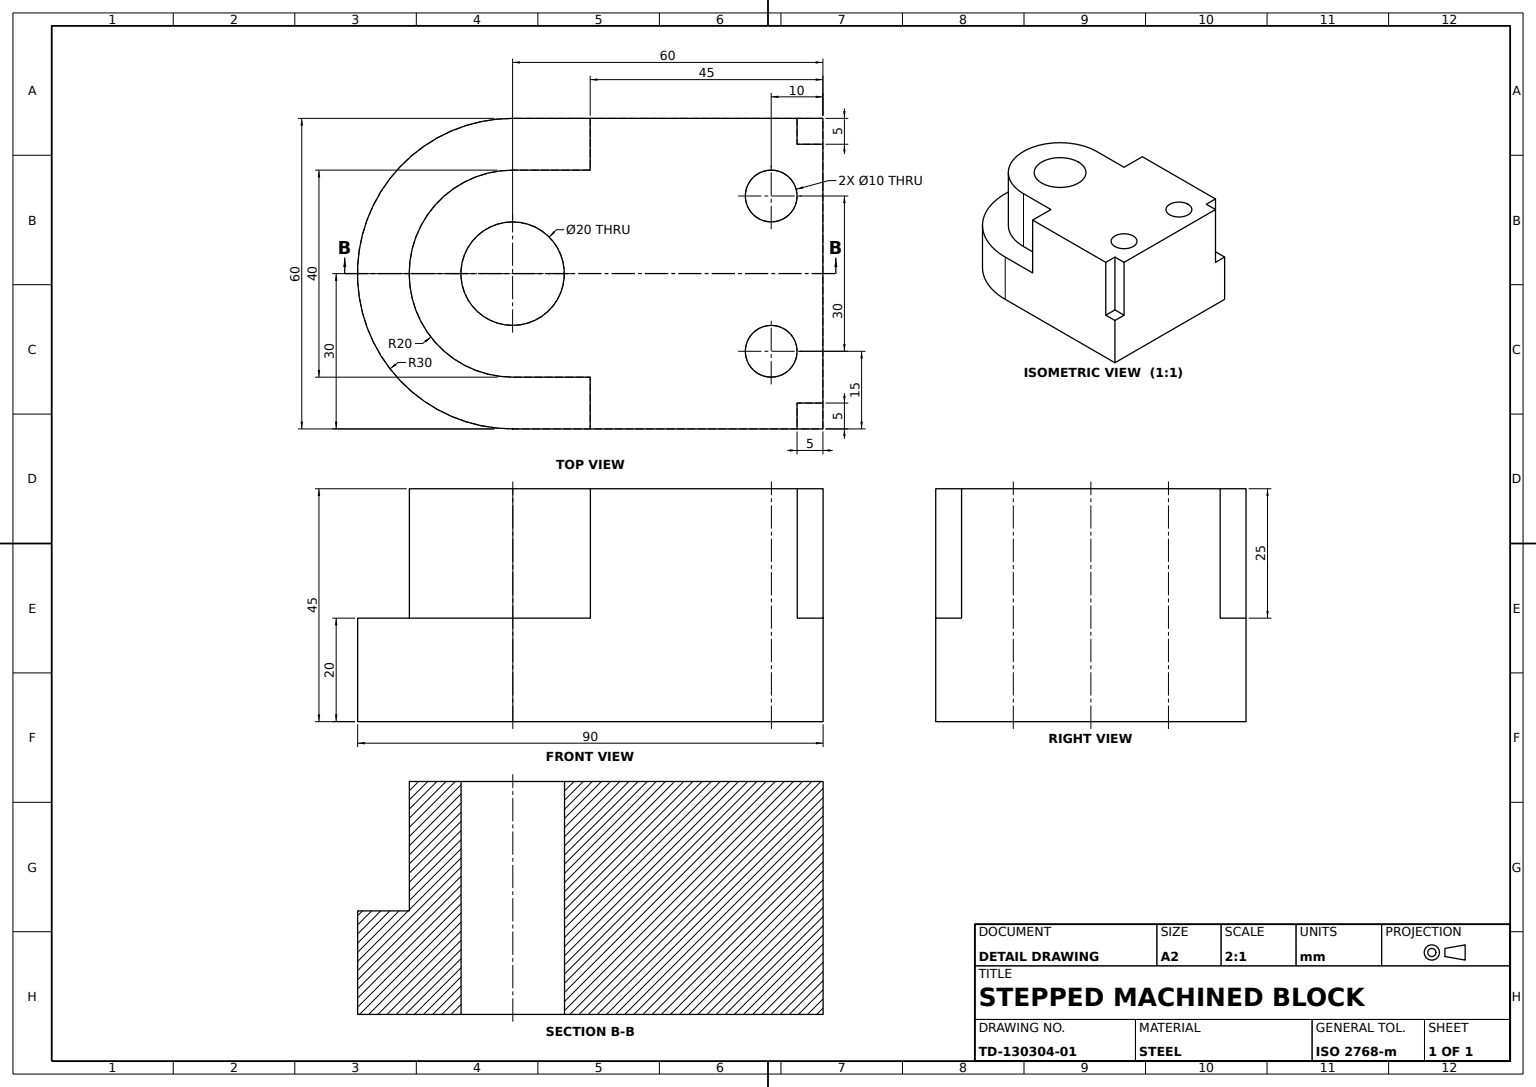
from build123d import *

# Parameters (mm, degrees)
BASE_BLOCK_DEPTH        = 20
STEP_PAD_1_DEPTH        = 5
STEP_START              = -5
STEP_PAD_2_DEPTH        = 5
ROUND_BOSS_SKETCH_R     = 20
ROUND_BOSS_DEPTH        = 20
RISER_BLOCK_1_DEPTH     = 20
SIDE_PAD_1_SKETCH_W     = 40
SIDE_PAD_1_SKETCH_H     = 10
SIDE_PAD_1_DEPTH        = 5
RISER_BLOCK_2_SKETCH_W  = 40
RISER_BLOCK_2_SKETCH_H  = 10
RISER_BLOCK_2_DEPTH     = 20
SIDE_PAD_2_SKETCH_W     = 40
SIDE_PAD_2_SKETCH_H     = 10
SIDE_PAD_2_DEPTH        = 5
RISER_BLOCK_3_SKETCH_W  = 40
RISER_BLOCK_3_SKETCH_H  = 10
RISER_BLOCK_3_DEPTH     = 20
BORE_20_SKETCH_R        = 10
BORE_20_DEPTH           = 76
CORNER_SLOT_1_SKETCH_W  = 5
CORNER_SLOT_1_SKETCH_H  = 5
CORNER_SLOT_1_5X5_DEPTH = 25
CORNER_SLOT_2_SKETCH_W  = 5
CORNER_SLOT_2_SKETCH_H  = 5
CORNER_SLOT_2_5X5_DEPTH = 25
HOLE_1_DEPTH            = 16
HOLE_1_DEPTH_BACK       = 53
HOLE_1_SKETCH_R         = 5
HOLE_2_SKETCH_R         = 5
HOLE_2_DEPTH            = 122
TOP_BLOCK_SKETCH_W      = 5
TOP_BLOCK_SKETCH_H      = 10
TOP_BLOCK_45_DEPTH      = 25


with BuildPart() as part:
    # Base Profile Sketch → Base Block (new body)
    with BuildSketch(Plane(origin=(0, 0, 0), x_dir=(1, 0, 0), z_dir=(0, 1, 0))):
        with BuildLine():
            Line((8.306767896, 1.392410292), (8.306767896, 31.392410292))
            Line((8.306767896, 31.392410292), (-51.693232104, 31.392410292))
            ThreePointArc((-51.693232104, 31.392410292), (-81.693232104, 1.392410292), (-51.693232104, -28.607589708))
            Line((-51.693232104, -28.607589708), (8.306767896, -28.607589708))
            Line((8.306767896, -28.607589708), (8.306767896, 1.392410292))
        make_face()
    extrude(amount=BASE_BLOCK_DEPTH)

    # Step Pad 1 Sketch → Step Pad 1 (add)
    with BuildSketch(Plane(origin=(0, 20, 0), x_dir=(1, 0, 0), z_dir=(0, 1, 0))):
        with BuildLine():
            ThreePointArc((-31.693232104, 1.392410292), (-37.55109648, 15.534545916), (-51.693232104, 21.392410292))
            ThreePointArc((-51.693232104, 21.392410292), (-71.693232104, 1.392410292), (-51.693232104, -18.607589708))
            ThreePointArc((-51.693232104, -18.607589708), (-37.55109648, -12.749725331), (-31.693232104, 1.392410292))
        make_face()
    extrude(amount=STEP_PAD_1_DEPTH)

    # Step Pad 2 Sketch → Step Pad 2 (add)
    with BuildSketch(Plane(origin=(0, 25, 0), x_dir=(1, 0, 0), z_dir=(0, 1, 0)).offset(STEP_START)):
        with BuildLine():
            Line((-51.693232104, 21.392410292), (8.306767896, 21.392410292))
            Line((8.306767896, 21.392410292), (8.306767896, -18.607589708))
            Line((8.306767896, -18.607589708), (-51.693232104, -18.607589708))
            ThreePointArc((-51.693232104, -18.607589708), (-71.693232104, 1.392410292), (-51.693232104, 21.392410292))
        make_face()
    extrude(amount=STEP_PAD_2_DEPTH)

    # Round Boss Sketch → Round Boss (add)
    with BuildSketch(Plane(origin=(0, 25, 0), x_dir=(1, 0, 0), z_dir=(0, 1, 0))):
        with Locations(Location((-51.693232104, 1.392410292, 0), (0, 0, 270))):
            Circle(ROUND_BOSS_SKETCH_R)
    extrude(amount=ROUND_BOSS_DEPTH)

    # Riser Block 1 Sketch → Riser Block 1 (add)
    with BuildSketch(Plane(origin=(0, 25, 0), x_dir=(1, 0, 0), z_dir=(0, 1, 0))):
        with BuildLine():
            Line((8.306767896, 21.392410292), (-51.693232104, 21.392410292))
            ThreePointArc((-51.693232104, 21.392410292), (-31.693232104, 1.392410292), (-51.693232104, -18.607589708))
            Line((-51.693232104, -18.607589708), (8.306767896, -18.607589708))
            Line((8.306767896, -18.607589708), (8.306767896, 21.392410292))
        make_face()
    extrude(amount=RISER_BLOCK_1_DEPTH)

    # Side Pad 1 Sketch → Side Pad 1 (add)
    with BuildSketch(Plane(origin=(0, 20, 0), x_dir=(1, 0, 0), z_dir=(0, 1, 0))):
        with Locations((-11.693232104, 26.392410292)):
            Rectangle(SIDE_PAD_1_SKETCH_W, SIDE_PAD_1_SKETCH_H)
    extrude(amount=SIDE_PAD_1_DEPTH)

    # Riser Block 2 Sketch → Riser Block 2 (add)
    with BuildSketch(Plane(origin=(0, 25, 0), x_dir=(1, 0, 0), z_dir=(0, 1, 0))):
        with Locations((-11.693232104, 26.392410292)):
            Rectangle(RISER_BLOCK_2_SKETCH_W, RISER_BLOCK_2_SKETCH_H)
    extrude(amount=RISER_BLOCK_2_DEPTH)

    # Side Pad 2 Sketch → Side Pad 2 (add)
    with BuildSketch(Plane(origin=(0, 20, 0), x_dir=(1, 0, 0), z_dir=(0, 1, 0))):
        with Locations((-11.693232104, -23.607589708)):
            Rectangle(SIDE_PAD_2_SKETCH_W, SIDE_PAD_2_SKETCH_H)
    extrude(amount=SIDE_PAD_2_DEPTH)

    # Riser Block 3 Sketch → Riser Block 3 (add)
    with BuildSketch(Plane(origin=(0, 25, 0), x_dir=(1, 0, 0), z_dir=(0, 1, 0))):
        with Locations((-11.693232104, -23.607589708)):
            Rectangle(RISER_BLOCK_3_SKETCH_W, RISER_BLOCK_3_SKETCH_H)
    extrude(amount=RISER_BLOCK_3_DEPTH)

    # Bore Ø20 Sketch → Bore Ø20 (cut)
    with BuildSketch(Plane(origin=(0, 45, 0), x_dir=(1, 0, 0), z_dir=(0, 1, 0))):
        with Locations(Location((-51.693232104, 1.392410292, 0), (0, 0, 270))):
            Circle(BORE_20_SKETCH_R)
    extrude(amount=-BORE_20_DEPTH, mode=Mode.SUBTRACT)

    # Corner Slot 1 Sketch → Corner Slot 1 5x5 (cut)
    with BuildSketch(Plane(origin=(0, 45, 0), x_dir=(1, 0, 0), z_dir=(0, 1, 0))):
        with Locations((5.806767896, 28.892410292)):
            Rectangle(CORNER_SLOT_1_SKETCH_W, CORNER_SLOT_1_SKETCH_H)
    extrude(amount=-CORNER_SLOT_1_5X5_DEPTH, mode=Mode.SUBTRACT)

    # Corner Slot 2 Sketch → Corner Slot 2 5x5 (cut)
    with BuildSketch(Plane(origin=(0, 45, 0), x_dir=(1, 0, 0), z_dir=(0, 1, 0))):
        with Locations((5.806767896, -26.107589708)):
            Rectangle(CORNER_SLOT_2_SKETCH_W, CORNER_SLOT_2_SKETCH_H)
    extrude(amount=-CORNER_SLOT_2_5X5_DEPTH, mode=Mode.SUBTRACT)

    # Hole 1 Sketch → Hole 1 (cut, two sides: drawn at the far end of the back side and taken through both)
    with BuildSketch(Plane(origin=(0, 45, 0), x_dir=(1, 0, 0), z_dir=(0, 1, 0)).offset(-HOLE_1_DEPTH_BACK)):
        with Locations(Location((-1.693232104, -13.607589708, 0), (0, 0, 270))):
            Circle(HOLE_1_SKETCH_R)
    extrude(amount=HOLE_1_DEPTH + HOLE_1_DEPTH_BACK, mode=Mode.SUBTRACT)

    # Hole 2 Sketch → Hole 2 (cut)
    with BuildSketch(Plane(origin=(0, 45, 0), x_dir=(1, 0, 0), z_dir=(0, 1, 0))):
        with Locations(Location((-1.693232104, 16.392410292, 0), (0, 0, 270))):
            Circle(HOLE_2_SKETCH_R)
    extrude(amount=-HOLE_2_DEPTH, mode=Mode.SUBTRACT)

    # Top Block Sketch → Top Block 45 (add)
    with BuildSketch(Plane(origin=(0, 20, 0), x_dir=(1, 0, 0), z_dir=(0, 1, 0))):
        with Locations((-34.193232104, 26.392410292)):
            Rectangle(TOP_BLOCK_SKETCH_W, TOP_BLOCK_SKETCH_H)
        with Locations((-34.193232104, -23.607589708)):
            Rectangle(TOP_BLOCK_SKETCH_W, TOP_BLOCK_SKETCH_H)
    extrude(amount=TOP_BLOCK_45_DEPTH)


solid = part.part
